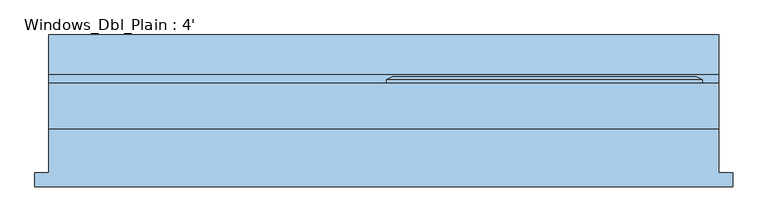
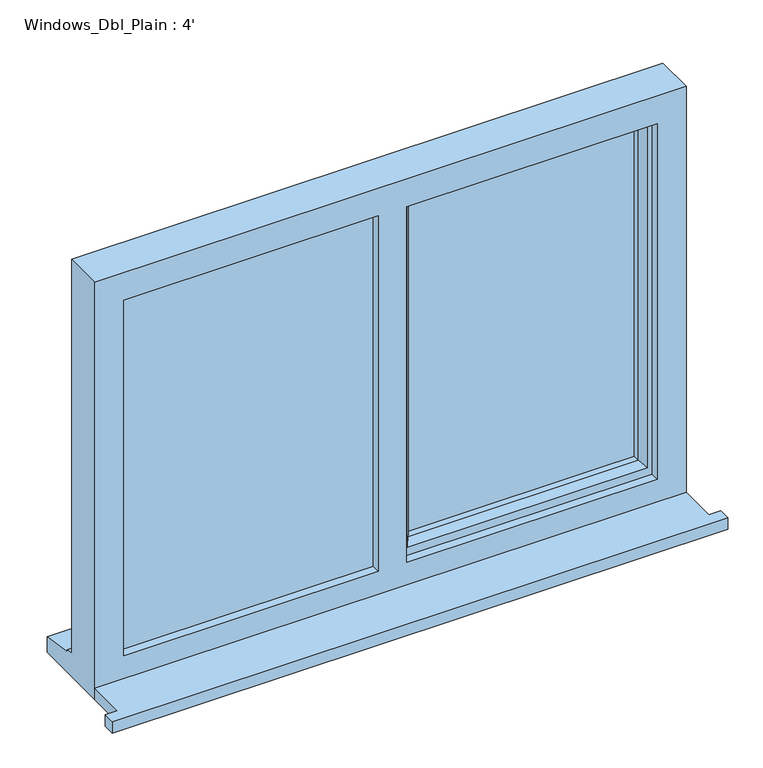
"""IFC4 building model written with IfcOpenShell, lengths in millimetres: window geometry, Windows_Dbl_Plain : 4'."""

from ifc_helpers import new_model, si_unit, frame, origin, place, context, project, spatial, polyline, outline, extrude, faceted_brep, source, transform, mapped, element, save


def windows_dbl_plain_4_905afcad(model_context):
    return source(origin(), model_context, "Body", "SolidModel", [
        extrude(outline(polyline([(-919.6, -123.2234322), (-919.6, -98.2234322), (-894.6, -98.2234322), (-894.6, -17.8634322), (324.6, -17.8634322), (324.6, -98.2234322), (349.6, -98.2234322), (349.6, -123.2234322), (-919.6, -123.2234322)])), frame((0.0, 0.0, 1200.0), z_axis=(0.0, 0.0, 1.0), x_axis=(1.0, 0.0, 0.0)), (0.0, 0.0, 1.0), 25.0),
        faceted_brep([(-280.0, 65.1365678, 2080.0), (-280.0, 70.9100705, 2080.0), (-280.0, 70.9100705, 1253.0), (-280.0, 65.1365678, 1253.0), (-270.0, 0.1365678, 2070.0), (-270.0, 65.1365678, 2070.0), (-270.0, 65.1365678, 1263.0), (-270.0, 0.1365678, 1263.0), (-230.0, 14.6294677, 2030.0), (-240.1480377, 0.1365678, 2040.1480377), (-240.1480377, 0.1365678, 1292.8519623), (-230.0, 14.6294677, 1303.0), (-230.0, 29.1365678, 2030.0), (-230.0, 29.1365678, 1303.0), (-240.0, 53.1365678, 2040.0), (-240.0, 29.1365678, 2040.0), (-240.0, 29.1365678, 1293.0), (-240.0, 53.1365678, 1293.0), (-230.0, 70.9100705, 2030.0), (-230.0, 53.1365678, 2030.0), (-230.0, 53.1365678, 1303.0), (-230.0, 70.9100705, 1303.0), (-247.4457548, 76.6835732, 2047.4457548), (-247.4457548, 76.6835732, 1285.5542452), (-269.2153903, 76.6835732, 2069.2153903), (-269.2153903, 76.6835732, 1263.7846097), (294.6, 70.9100705, 1253.0), (294.6, 65.1365678, 1253.0), (284.6, 65.1365678, 1263.0), (284.6, 0.1365678, 1263.0), (254.7480377, 0.1365678, 1292.8519623), (244.6, 14.6294677, 1303.0), (244.6, 29.1365678, 1303.0), (254.6, 29.1365678, 1293.0), (254.6, 53.1365678, 1293.0), (244.6, 53.1365678, 1303.0), (244.6, 70.9100705, 1303.0), (262.0457548, 76.6835732, 1285.5542452), (283.8153903, 76.6835732, 1263.7846097), (294.6, 70.9100705, 2080.0), (294.6, 65.1365678, 2080.0), (284.6, 65.1365678, 2070.0), (284.6, 0.1365678, 2070.0), (254.7480377, 0.1365678, 2040.1480377), (244.6, 14.6294677, 2030.0), (244.6, 29.1365678, 2030.0), (254.6, 29.1365678, 2040.0), (254.6, 53.1365678, 2040.0), (244.6, 53.1365678, 2030.0), (244.6, 70.9100705, 2030.0), (262.0457548, 76.6835732, 2047.4457548), (283.8153903, 76.6835732, 2069.2153903)], [[[0, 1, 2, 3]], [[4, 5, 6, 7]], [[8, 9, 10, 11]], [[12, 8, 11, 13]], [[14, 15, 16, 17]], [[18, 19, 20, 21]], [[22, 18, 21, 23]], [[1, 24, 25, 2]], [[3, 2, 26, 27]], [[7, 6, 28, 29]], [[11, 10, 30, 31]], [[13, 11, 31, 32]], [[17, 16, 33, 34]], [[21, 20, 35, 36]], [[23, 21, 36, 37]], [[2, 25, 38, 26]], [[27, 26, 39, 40]], [[29, 28, 41, 42]], [[31, 30, 43, 44]], [[32, 31, 44, 45]], [[34, 33, 46, 47]], [[36, 35, 48, 49]], [[37, 36, 49, 50]], [[26, 38, 51, 39]], [[40, 39, 1, 0]], [[3, 27, 40, 0], [5, 41, 28, 6]], [[42, 41, 5, 4]], [[7, 29, 42, 4], [9, 43, 30, 10]], [[44, 43, 9, 8]], [[45, 44, 8, 12]], [[15, 46, 33, 16], [13, 32, 45, 12]], [[47, 46, 15, 14]], [[17, 34, 47, 14], [19, 48, 35, 20]], [[49, 48, 19, 18]], [[50, 49, 18, 22]], [[24, 51, 38, 25], [23, 37, 50, 22]], [[39, 51, 24, 1]]]),
        extrude(outline(polyline([(2050.0, -310.0), (2070.0, -310.0), (2070.0, -854.6), (1263.0, -854.6), (1263.0, -310.0), (1283.0, -310.0), (1283.0, -834.6), (2050.0, -834.6), (2050.0, -310.0)])), frame((0.0, 24.1365678, 0.0), z_axis=(0.0, 1.0, 0.0), x_axis=(0.0, 0.0, 1.0)), (0.0, 0.0, 1.0), 41.0),
        faceted_brep([(324.6, -17.8634322, 2110.0), (-894.6, -17.8634322, 2110.0), (-894.6, -17.8634322, 1200.0), (324.6, -17.8634322, 1200.0), (264.6, -17.8634322, 2050.0), (264.6, -17.8634322, 1275.0), (-252.0, -17.8634322, 1275.0), (-252.0, -17.8634322, 2050.0), (-310.0, -17.8634322, 2050.0), (-310.0, -17.8634322, 1275.0), (-834.6, -17.8634322, 1275.0), (-834.6, -17.8634322, 2050.0), (-894.6, 65.1365678, 2110.0), (-894.6, 65.1365678, 1251.0), (-894.6, 80.1365678, 1249.68767), (-894.6, 80.1365678, 1244.7449676), (-894.6, 152.6365678, 1233.8088847), (-894.6, 152.6365678, 1200.0), (324.6, 65.1365678, 2110.0), (324.6, 65.1365678, 1251.0), (-854.6, 65.1365678, 2070.0), (-854.6, 65.1365678, 1263.0), (-310.0, 65.1365678, 1263.0), (-310.0, 65.1365678, 2070.0), (-270.0, 65.1365678, 2070.0), (-270.0, 65.1365678, 1263.0), (284.6, 65.1365678, 1263.0), (284.6, 65.1365678, 2070.0), (-854.6, 0.1365678, 2070.0), (-854.6, 0.1365678, 1263.0), (-300.0, 0.1365678, 2070.0), (-300.0, 0.1365678, 1263.0), (-310.0, 0.1365678, 2050.0), (-834.6, 0.1365678, 2050.0), (-834.6, 0.1365678, 1275.0), (-310.0, 0.1365678, 1275.0), (-270.0, 0.1365678, 2070.0), (284.6, 0.1365678, 2070.0), (284.6, 0.1365678, 1263.0), (-270.0, 0.1365678, 1263.0), (264.6, 0.1365678, 2050.0), (-252.0, 0.1365678, 2050.0), (-252.0, 0.1365678, 1275.0), (264.6, 0.1365678, 1275.0), (-310.0, 24.1365678, 2070.0), (-300.0, 24.1365678, 2070.0), (324.6, 152.6365678, 1200.0), (324.6, 152.6365678, 1233.8088847), (324.6, 80.1365678, 1244.7449676), (324.6, 80.1365678, 1249.68767), (-300.0, 24.1365678, 1263.0), (-310.0, 24.1365678, 1263.0)], [[[0, 1, 2, 3], [4, 5, 6, 7], [8, 9, 10, 11]], [[2, 1, 12, 13, 14, 15, 16, 17]], [[13, 12, 18, 19], [20, 21, 22, 23], [24, 25, 26, 27]], [[21, 20, 28, 29]], [[28, 30, 31, 29], [32, 33, 34, 35]], [[36, 37, 38, 39], [40, 41, 42, 43]], [[33, 11, 10, 34]], [[1, 0, 18, 12]], [[28, 20, 23, 44, 45, 30]], [[27, 37, 36, 24]], [[11, 33, 32, 8]], [[40, 4, 7, 41]], [[19, 18, 0, 3, 46, 47, 48, 49]], [[27, 26, 38, 37]], [[4, 40, 43, 5]], [[45, 50, 31, 30]], [[50, 45, 44, 51]], [[51, 44, 23, 22]], [[25, 24, 36, 39]], [[41, 7, 6, 42]], [[8, 32, 35, 9]], [[46, 3, 2, 17]], [[47, 46, 17, 16]], [[48, 47, 16, 15]], [[49, 48, 15, 14]], [[19, 49, 14, 13]], [[22, 21, 29, 31, 50, 51]], [[26, 25, 39, 38]], [[6, 5, 43, 42]], [[35, 34, 10, 9]]]),
        extrude(outline(polyline([(-854.6, 24.1365678), (-300.0, 24.1365678), (-300.0, 0.1365678), (-854.6, 0.1365678), (-854.6, 24.1365678)])), frame((0.0, 0.0, 1263.0), z_axis=(0.0, 0.0, 1.0), x_axis=(1.0, 0.0, 0.0)), (0.0, 0.0, 1.0), 807.0),
        extrude(outline(polyline([(254.6, 29.1365678), (-240.0, 29.1365678), (-240.0, 53.1365678), (254.6, 53.1365678), (254.6, 29.1365678)])), frame((0.0, 0.0, 1293.0), z_axis=(0.0, 0.0, 1.0), x_axis=(1.0, 0.0, 0.0)), (0.0, 0.0, 1.0), 747.0),
    ])


if __name__ == "__main__":
    model = new_model("IFC4")
    model_context = context("Model", 3, world=origin())
    ifc_project = project(units=[si_unit("LENGTHUNIT", "METRE", prefix="MILLI")], contexts=[model_context])
    site = spatial("IfcSite", under=ifc_project)
    building = spatial("IfcBuilding", under=site)
    placement = place(None, origin())
    windows_dbl_plain_4_shape = windows_dbl_plain_4_905afcad(model_context)
    element("IfcWindow", 1, ObjectType="Windows_Dbl_Plain : 4'", at=placement, inside=building, context=model_context, shape_type="MappedRepresentation", body=[
        mapped(windows_dbl_plain_4_shape, transform((0.0, 0.0, 0.0), x_axis=(1.0, 0.0, 0.0), y_axis=(0.0, 1.0, 0.0), z_axis=(0.0, 0.0, 1.0))),
    ])
    save(model, "model.ifc")

# Revit data of these elements
# Type "Windows_Dbl_Plain : 4'"
#   Type Mark = "56"
#   Operation = "DoublePanelVertical"
#   Construction Type Id = "GSP4R"
#   Manufacturer = "Revit"
#   Keynote = "L10"
#   Analytic Construction = "1/8 in Pilkington single glazing"
#   Wrap Layers (Ext) from Ext = 0.336286 ft
#   Wrap Layers (Int) from Ext = 0.582349 ft
#   Window Board Projection = 0.082021 ft
#   Window Board Extension = 0.082021 ft
#   Visual Light Transmittance = 0.9
#   Solar Heat Gain Coefficient = 0.78
#   Rough Width = 4.0 ft
#   Rough Height = 2.985564 ft
#   Height = 2.985564 ft
#   Width = 4.0 ft
#   Heat Transfer Coefficient (U) = 3.6886 W/(m²·K)
#   Glazing Thickness = 0.07874 ft
#   FrameOffset - External = 0.164042 ft
#   Frame Depth = 0.213255 ft
#   Default Head Height = 6.922572 ft
#   Cill Depth = 0.287073 ft
#   Cavity Closer Width = 0.164042 ft
#   Cavity Closer Offset from Ext = 0.336286 ft
#   Cavity Closer Depth = 0.278871 ft
#   Vis - Cavity Closers = yes
#   Define Thermal Properties by = 1
#   Material Trim = Window Frame
#   Material Glass = Glass
#   Material Frame = Window Frame
#   Wall Closure = (empty or 0)
# Element 1 (IfcWindow, "Windows_Dbl_Plain : 4'")
#   Materials on its faces: "Window Frame", "Glass"
# Materials
#   "Window Frame": colour RGB 249 249 249, transparency 0, Keynote = "L10", Cost = 0
#   "Glass": class "Glass", colour RGB 0 128 192, transparency 0.9, Description = "Soda Lime Glass", Cost = 0
